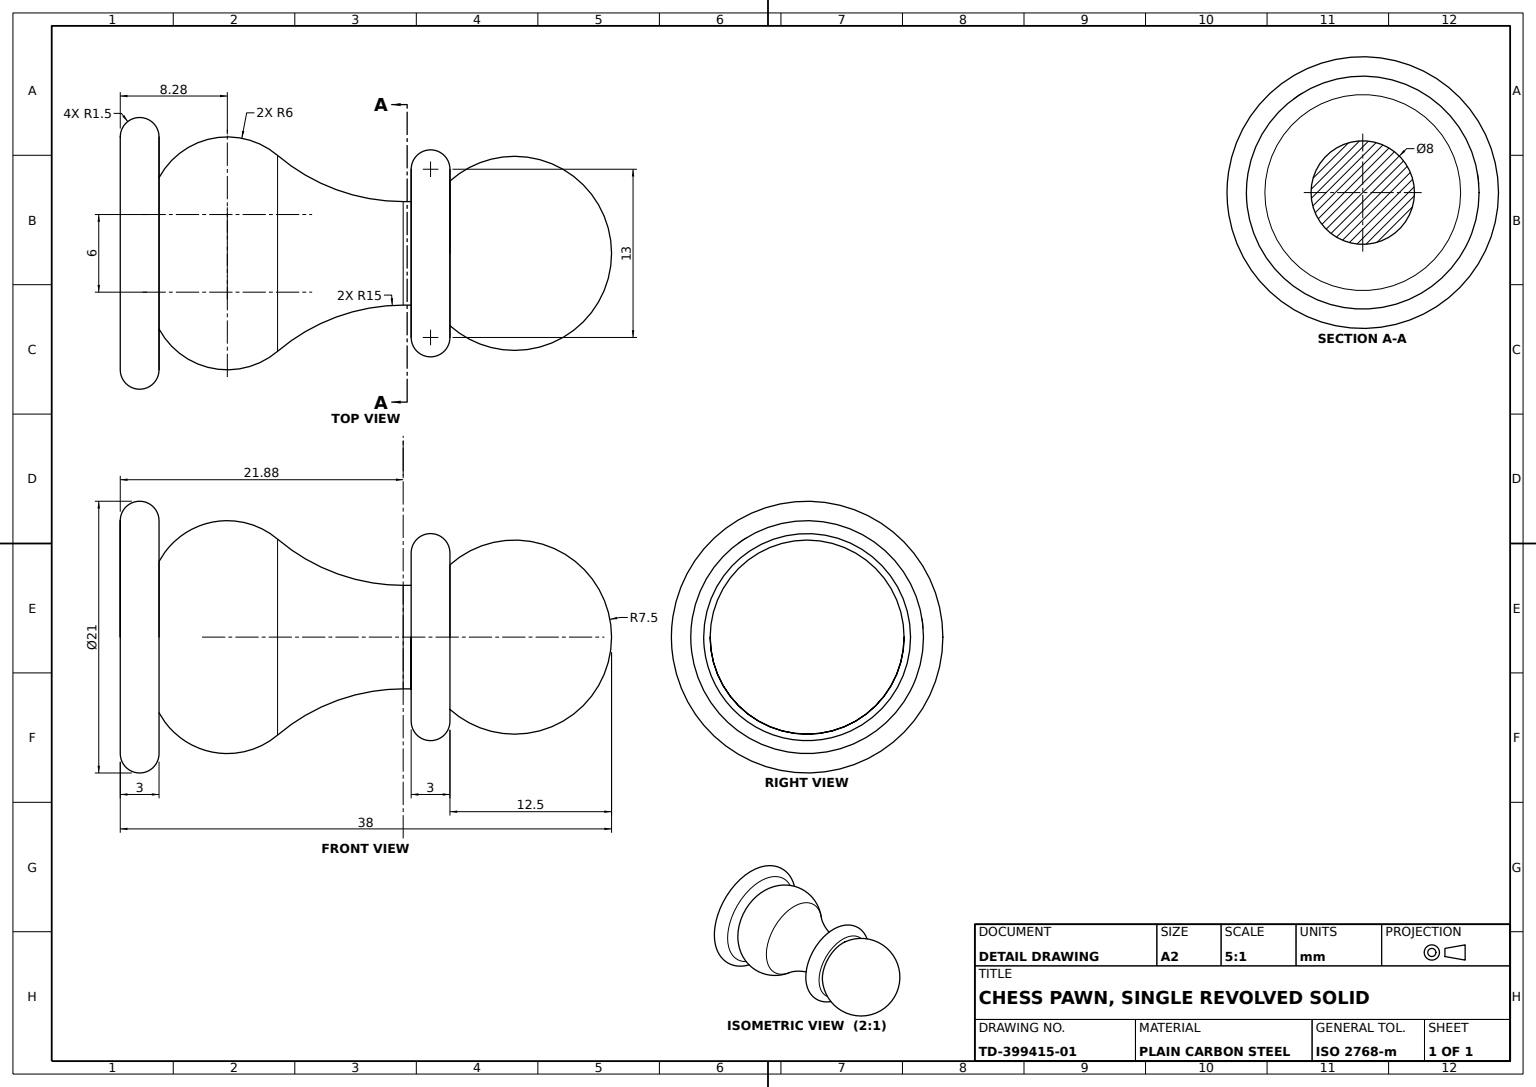
from build123d import *


with BuildPart() as part:
    # Pawn Profile Sketch → Pawn Body Revolve (revolve)
    with BuildSketch(Plane.XY, mode=Mode.PRIVATE) as pawn_body_revolve_sk:
        with BuildLine():
            Line((0, -15.5), (0, -12.5))
            Line((0, -12.5), (-5.590169944, -12.5))
            Line((-5.590169944, -12.5), (-6.5, -12.5))
            ThreePointArc((-6.5, -12.5), (-8, -14), (-6.5, -15.5))
            Line((-6.5, -15.5), (-4, -15.5))
            Line((-4, -15.5), (0, -15.5))
        make_face()
        with BuildLine():
            Line((0, -12.5), (0, 0))
            ThreePointArc((0, 0), (-6.846531969, -4.438137822), (-5.590169944, -12.5))
            Line((-5.590169944, -12.5), (0, -12.5))
        make_face()
        with BuildLine():
            Line((0, -34.915148474), (0, -15.5))
            Line((0, -15.5), (-4, -15.5))
            Line((-4, -15.5), (-4, -16.117525543))
            ThreePointArc((-4, -16.117525543), (-4.921140468, -21.293017238), (-7.571428571, -25.83286162))
            ThreePointArc((-7.571428571, -25.83286162), (-8.896695439, -30.827591061), (-5.847981266, -35))
            Line((-5.847981266, -35), (-0.152018734, -35))
            ThreePointArc((-0.152018734, -35), (-0.075701594, -34.958125638), (0, -34.915148474))
        make_face()
        with BuildLine():
            Line((0, -38), (0, -35))
            Line((0, -35), (-0.152018734, -35))
            Line((-0.152018734, -35), (-5.847981266, -35))
            Line((-5.847981266, -35), (-9, -35))
            ThreePointArc((-9, -35), (-10.5, -36.5), (-9, -38))
            Line((-9, -38), (0, -38))
        make_face()
    revolve(pawn_body_revolve_sk.sketch.rotate(Axis((0, 0, 0), (0, -1, 0)), 270), axis=Axis((0, 0, 0), (0, -1, 0)))


solid = part.part
